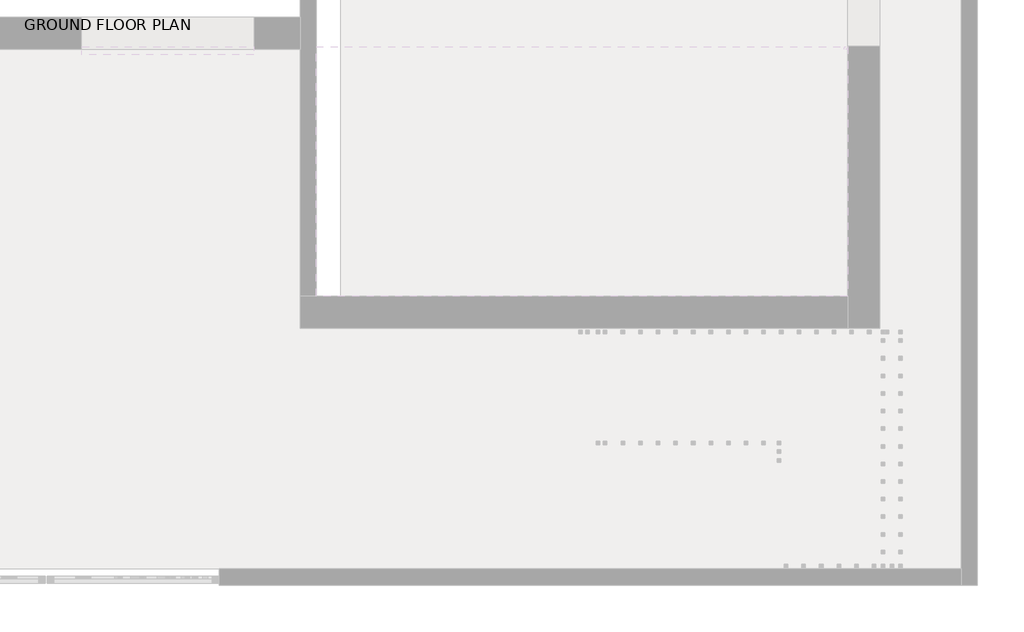
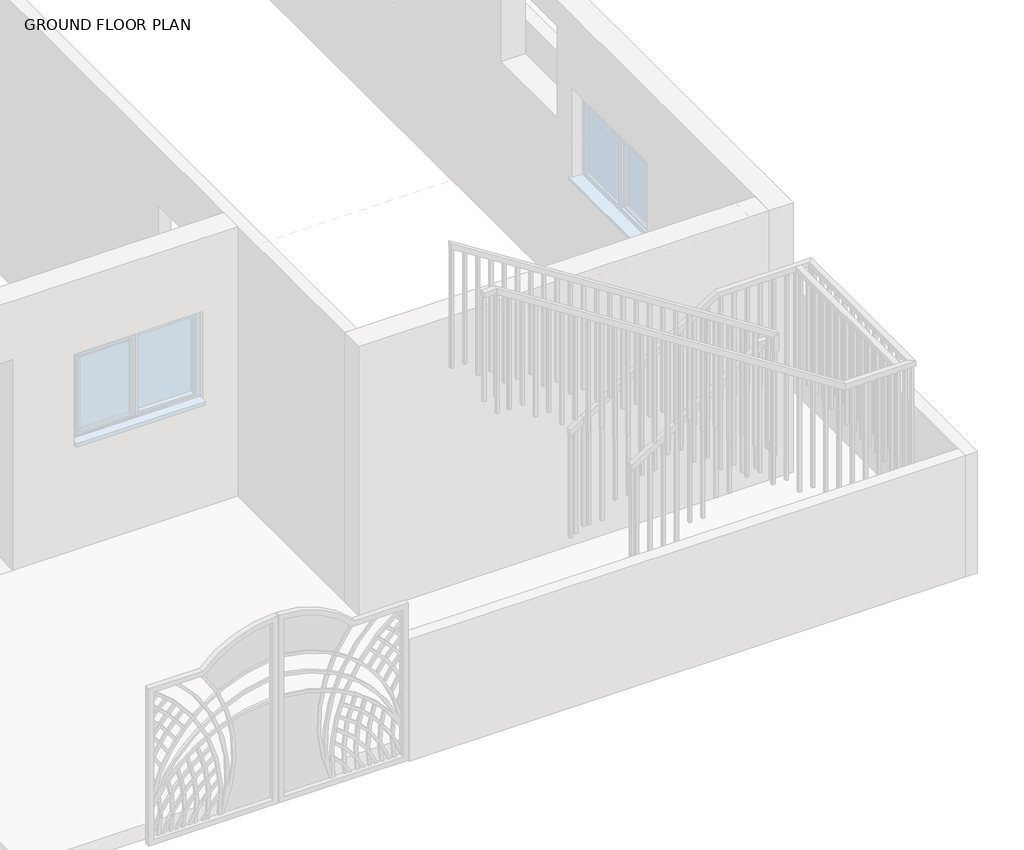
# One storey, part 12 of 23: 2 railings.
"""IFC4 building model written with IfcOpenShell, lengths in millimetres."""

from ifc_helpers import new_model, si_unit, frame, origin, place, context, project, spatial, polyline, outline, extrude, faceted_brep, element, save

model = new_model("IFC4")

# Units and contexts
model_context = context("Model", 3, world=origin())
ifc_project = project(units=[si_unit("LENGTHUNIT", "METRE", prefix="MILLI")], contexts=[model_context])

# Site, building, storey
site = spatial("IfcSite", under=ifc_project)
building = spatial("IfcBuilding", under=site)
storey = spatial("IfcBuildingStorey", under=building, Name="GROUND FLOOR PLAN", Elevation=487.68)

# Railings
placement = place(None, origin())
element("IfcRailing", 1, ObjectType="1100mm", at=placement, inside=storey, context=model_context, shape_type="SolidModel", body=[
    faceted_brep([(-8805.870786, -10220.0521308, 1832.3649576), (-8805.870786, -10220.0521308, 1773.007357), (-8805.870786, -10270.0521308, 1773.007357), (-8805.870786, -10270.0521308, 1832.3649576), (-7409.7306254, -10220.0521308, 2725.6), (-7395.1045513, -10220.0521308, 2675.6), (-7395.1045513, -10270.0521308, 2675.6), (-7409.7306254, -10270.0521308, 2725.6), (-6621.5344696, -10220.0521308, 2725.6), (-6621.5344696, -10220.0521308, 2675.6), (-6671.5344696, -10270.0521308, 2675.6), (-6671.5344696, -10270.0521308, 2725.6), (-6621.5344696, -11933.6860066, 2725.6), (-6621.5344696, -11933.6860066, 2675.6), (-6671.5344696, -11883.6860066, 2675.6), (-6671.5344696, -11883.6860066, 2725.6), (-7155.718398, -11933.6860066, 2725.6), (-7170.3479429, -11933.6860066, 2675.6), (-7170.3479429, -11883.6860066, 2675.6), (-7155.718398, -11883.6860066, 2725.6), (-10457.8773536, -11933.6860066, 4838.88), (-10472.5068984, -11933.6860066, 4788.88), (-10472.5068984, -11883.6860066, 4788.88), (-10457.8773536, -11883.6860066, 4838.88), (-10583.5985666, -11933.6860066, 4838.88), (-10583.5985666, -11883.6860066, 4838.88), (-10583.5985666, -11883.6860066, 4788.88), (-10583.5985666, -11933.6860066, 4788.88)], [[[0, 1, 2, 3]], [[1, 0, 4, 5]], [[2, 1, 5, 6]], [[3, 2, 6, 7]], [[0, 3, 7, 4]], [[5, 4, 8, 9]], [[6, 5, 9, 10]], [[7, 6, 10, 11]], [[4, 7, 11, 8]], [[9, 8, 12, 13]], [[10, 9, 13, 14]], [[11, 10, 14, 15]], [[8, 11, 15, 12]], [[13, 12, 16, 17]], [[14, 13, 17, 18]], [[15, 14, 18, 19]], [[12, 15, 19, 16]], [[17, 16, 20, 21]], [[18, 17, 21, 22]], [[19, 18, 22, 23]], [[16, 19, 23, 20]], [[24, 25, 26, 27]], [[21, 20, 24, 27]], [[22, 21, 27, 26]], [[23, 22, 26, 25]], [[20, 23, 25, 24]]]),
    extrude(outline(polyline([(-10446.5344696, -11921.1860066), (-10471.5344696, -11921.1860066), (-10471.5344696, -11896.1860066), (-10446.5344696, -11896.1860066), (-10446.5344696, -11921.1860066)])), frame((0.0, 0.0, 3738.88), z_axis=(0.0, 0.0, 1.0), x_axis=(1.0, 0.0, 0.0)), (0.0, 0.0, 1.0), 1050.0),
    extrude(outline(polyline([(4692.2622966, -10321.5344696), (4708.2615264, -10346.5344696), (3576.32, -10346.5344696), (3576.32, -10321.5344696), (4692.2622966, -10321.5344696)])), frame((0.0, -11921.1860066, 0.0), z_axis=(0.0, 1.0, 0.0), x_axis=(0.0, 0.0, 1.0)), (0.0, 0.0, 1.0), 25.0),
    extrude(outline(polyline([(4612.2661476, -10196.5344696), (4628.2653774, -10221.5344696), (3576.32, -10221.5344696), (3576.32, -10196.5344696), (4612.2661476, -10196.5344696)])), frame((0.0, -11921.1860066, 0.0), z_axis=(0.0, 1.0, 0.0), x_axis=(0.0, 0.0, 1.0)), (0.0, 0.0, 1.0), 25.0),
    extrude(outline(polyline([(4532.2699985, -10071.5344696), (4548.2692283, -10096.5344696), (3413.76, -10096.5344696), (3413.76, -10071.5344696), (4532.2699985, -10071.5344696)])), frame((0.0, -11921.1860066, 0.0), z_axis=(0.0, 1.0, 0.0), x_axis=(0.0, 0.0, 1.0)), (0.0, 0.0, 1.0), 25.0),
    extrude(outline(polyline([(4452.2738495, -9946.5344696), (4468.2730793, -9971.5344696), (3413.76, -9971.5344696), (3413.76, -9946.5344696), (4452.2738495, -9946.5344696)])), frame((0.0, -11921.1860066, 0.0), z_axis=(0.0, 1.0, 0.0), x_axis=(0.0, 0.0, 1.0)), (0.0, 0.0, 1.0), 25.0),
    extrude(outline(polyline([(4372.2777004, -9821.5344696), (4388.2769302, -9846.5344696), (3251.2, -9846.5344696), (3251.2, -9821.5344696), (4372.2777004, -9821.5344696)])), frame((0.0, -11921.1860066, 0.0), z_axis=(0.0, 1.0, 0.0), x_axis=(0.0, 0.0, 1.0)), (0.0, 0.0, 1.0), 25.0),
    extrude(outline(polyline([(4292.2815514, -9696.5344696), (4308.2807812, -9721.5344696), (3251.2, -9721.5344696), (3251.2, -9696.5344696), (4292.2815514, -9696.5344696)])), frame((0.0, -11921.1860066, 0.0), z_axis=(0.0, 1.0, 0.0), x_axis=(0.0, 0.0, 1.0)), (0.0, 0.0, 1.0), 25.0),
    extrude(outline(polyline([(4212.2854023, -9571.5344696), (4228.2846321, -9596.5344696), (3088.64, -9596.5344696), (3088.64, -9571.5344696), (4212.2854023, -9571.5344696)])), frame((0.0, -11921.1860066, 0.0), z_axis=(0.0, 1.0, 0.0), x_axis=(0.0, 0.0, 1.0)), (0.0, 0.0, 1.0), 25.0),
    extrude(outline(polyline([(4132.2892533, -9446.5344696), (4148.2884831, -9471.5344696), (3088.64, -9471.5344696), (3088.64, -9446.5344696), (4132.2892533, -9446.5344696)])), frame((0.0, -11921.1860066, 0.0), z_axis=(0.0, 1.0, 0.0), x_axis=(0.0, 0.0, 1.0)), (0.0, 0.0, 1.0), 25.0),
    extrude(outline(polyline([(4052.2931042, -9321.5344696), (4068.292334, -9346.5344696), (2926.08, -9346.5344696), (2926.08, -9321.5344696), (4052.2931042, -9321.5344696)])), frame((0.0, -11921.1860066, 0.0), z_axis=(0.0, 1.0, 0.0), x_axis=(0.0, 0.0, 1.0)), (0.0, 0.0, 1.0), 25.0),
    extrude(outline(polyline([(3972.2969552, -9196.5344696), (3988.296185, -9221.5344696), (2926.08, -9221.5344696), (2926.08, -9196.5344696), (3972.2969552, -9196.5344696)])), frame((0.0, -11921.1860066, 0.0), z_axis=(0.0, 1.0, 0.0), x_axis=(0.0, 0.0, 1.0)), (0.0, 0.0, 1.0), 25.0),
    extrude(outline(polyline([(3892.3008061, -9071.5344696), (3908.3000359, -9096.5344696), (2763.52, -9096.5344696), (2763.52, -9071.5344696), (3892.3008061, -9071.5344696)])), frame((0.0, -11921.1860066, 0.0), z_axis=(0.0, 1.0, 0.0), x_axis=(0.0, 0.0, 1.0)), (0.0, 0.0, 1.0), 25.0),
    extrude(outline(polyline([(3812.3046571, -8946.5344696), (3828.3038869, -8971.5344696), (2763.52, -8971.5344696), (2763.52, -8946.5344696), (3812.3046571, -8946.5344696)])), frame((0.0, -11921.1860066, 0.0), z_axis=(0.0, 1.0, 0.0), x_axis=(0.0, 0.0, 1.0)), (0.0, 0.0, 1.0), 25.0),
    extrude(outline(polyline([(3732.308508, -8821.5344696), (3748.3077378, -8846.5344696), (2600.96, -8846.5344696), (2600.96, -8821.5344696), (3732.308508, -8821.5344696)])), frame((0.0, -11921.1860066, 0.0), z_axis=(0.0, 1.0, 0.0), x_axis=(0.0, 0.0, 1.0)), (0.0, 0.0, 1.0), 25.0),
    extrude(outline(polyline([(3652.312359, -8696.5344696), (3668.3115888, -8721.5344696), (2600.96, -8721.5344696), (2600.96, -8696.5344696), (3652.312359, -8696.5344696)])), frame((0.0, -11921.1860066, 0.0), z_axis=(0.0, 1.0, 0.0), x_axis=(0.0, 0.0, 1.0)), (0.0, 0.0, 1.0), 25.0),
    extrude(outline(polyline([(3572.3162099, -8571.5344696), (3588.3154397, -8596.5344696), (2438.4, -8596.5344696), (2438.4, -8571.5344696), (3572.3162099, -8571.5344696)])), frame((0.0, -11921.1860066, 0.0), z_axis=(0.0, 1.0, 0.0), x_axis=(0.0, 0.0, 1.0)), (0.0, 0.0, 1.0), 25.0),
    extrude(outline(polyline([(3492.3200609, -8446.5344696), (3508.3192907, -8471.5344696), (2438.4, -8471.5344696), (2438.4, -8446.5344696), (3492.3200609, -8446.5344696)])), frame((0.0, -11921.1860066, 0.0), z_axis=(0.0, 1.0, 0.0), x_axis=(0.0, 0.0, 1.0)), (0.0, 0.0, 1.0), 25.0),
    extrude(outline(polyline([(3412.3239118, -8321.5344696), (3428.3231416, -8346.5344696), (2275.84, -8346.5344696), (2275.84, -8321.5344696), (3412.3239118, -8321.5344696)])), frame((0.0, -11921.1860066, 0.0), z_axis=(0.0, 1.0, 0.0), x_axis=(0.0, 0.0, 1.0)), (0.0, 0.0, 1.0), 25.0),
    extrude(outline(polyline([(3332.3277628, -8196.5344696), (3348.3269926, -8221.5344696), (2275.84, -8221.5344696), (2275.84, -8196.5344696), (3332.3277628, -8196.5344696)])), frame((0.0, -11921.1860066, 0.0), z_axis=(0.0, 1.0, 0.0), x_axis=(0.0, 0.0, 1.0)), (0.0, 0.0, 1.0), 25.0),
    extrude(outline(polyline([(3252.3316137, -8071.5344696), (3268.3308435, -8096.5344696), (2113.28, -8096.5344696), (2113.28, -8071.5344696), (3252.3316137, -8071.5344696)])), frame((0.0, -11921.1860066, 0.0), z_axis=(0.0, 1.0, 0.0), x_axis=(0.0, 0.0, 1.0)), (0.0, 0.0, 1.0), 25.0),
    extrude(outline(polyline([(3172.3354647, -7946.5344696), (3188.3346945, -7971.5344696), (2113.28, -7971.5344696), (2113.28, -7946.5344696), (3172.3354647, -7946.5344696)])), frame((0.0, -11921.1860066, 0.0), z_axis=(0.0, 1.0, 0.0), x_axis=(0.0, 0.0, 1.0)), (0.0, 0.0, 1.0), 25.0),
    extrude(outline(polyline([(3092.4129874, -7821.5344696), (3108.4077111, -7846.5344696), (1950.72, -7846.5344696), (1950.72, -7821.5344696), (3092.4129874, -7821.5344696)])), frame((0.0, -11921.1860066, 0.0), z_axis=(0.0, 1.0, 0.0), x_axis=(0.0, 0.0, 1.0)), (0.0, 0.0, 1.0), 25.0),
    extrude(outline(polyline([(3012.4393691, -7696.5344696), (3028.4340928, -7721.5344696), (1950.72, -7721.5344696), (1950.72, -7696.5344696), (3012.4393691, -7696.5344696)])), frame((0.0, -11921.1860066, 0.0), z_axis=(0.0, 1.0, 0.0), x_axis=(0.0, 0.0, 1.0)), (0.0, 0.0, 1.0), 25.0),
    extrude(outline(polyline([(2932.4657508, -7571.5344696), (2948.4604745, -7596.5344696), (1788.16, -7596.5344696), (1788.16, -7571.5344696), (2932.4657508, -7571.5344696)])), frame((0.0, -11921.1860066, 0.0), z_axis=(0.0, 1.0, 0.0), x_axis=(0.0, 0.0, 1.0)), (0.0, 0.0, 1.0), 25.0),
    extrude(outline(polyline([(2852.4921325, -7446.5344696), (2868.4868562, -7471.5344696), (1788.16, -7471.5344696), (1788.16, -7446.5344696), (2852.4921325, -7446.5344696)])), frame((0.0, -11921.1860066, 0.0), z_axis=(0.0, 1.0, 0.0), x_axis=(0.0, 0.0, 1.0)), (0.0, 0.0, 1.0), 25.0),
    extrude(outline(polyline([(2772.3547194, -7321.5344696), (2788.3539492, -7346.5344696), (1625.6, -7346.5344696), (1625.6, -7321.5344696), (2772.3547194, -7321.5344696)])), frame((0.0, -11921.1860066, 0.0), z_axis=(0.0, 1.0, 0.0), x_axis=(0.0, 0.0, 1.0)), (0.0, 0.0, 1.0), 25.0),
    extrude(outline(polyline([(2692.3585703, -7196.5344696), (2708.3578001, -7221.5344696), (1625.6, -7221.5344696), (1625.6, -7196.5344696), (2692.3585703, -7196.5344696)])), frame((0.0, -11921.1860066, 0.0), z_axis=(0.0, 1.0, 0.0), x_axis=(0.0, 0.0, 1.0)), (0.0, 0.0, 1.0), 25.0),
    extrude(outline(polyline([(-7071.5344696, -11921.1860066), (-7096.5344696, -11921.1860066), (-7096.5344696, -11896.1860066), (-7071.5344696, -11896.1860066), (-7071.5344696, -11921.1860066)])), frame((0.0, 0.0, 1625.6), z_axis=(0.0, 0.0, 1.0), x_axis=(1.0, 0.0, 0.0)), (0.0, 0.0, 1.0), 1050.0),
    extrude(outline(polyline([(-6946.5344696, -11921.1860066), (-6971.5344696, -11921.1860066), (-6971.5344696, -11896.1860066), (-6946.5344696, -11896.1860066), (-6946.5344696, -11921.1860066)])), frame((0.0, 0.0, 1625.6), z_axis=(0.0, 0.0, 1.0), x_axis=(1.0, 0.0, 0.0)), (0.0, 0.0, 1.0), 1050.0),
    extrude(outline(polyline([(-6821.5344696, -11921.1860066), (-6846.5344696, -11921.1860066), (-6846.5344696, -11896.1860066), (-6821.5344696, -11896.1860066), (-6821.5344696, -11921.1860066)])), frame((0.0, 0.0, 1625.6), z_axis=(0.0, 0.0, 1.0), x_axis=(1.0, 0.0, 0.0)), (0.0, 0.0, 1.0), 1050.0),
    extrude(outline(polyline([(-6696.5344696, -11921.1860066), (-6721.5344696, -11921.1860066), (-6721.5344696, -11896.1860066), (-6696.5344696, -11896.1860066), (-6696.5344696, -11921.1860066)])), frame((0.0, 0.0, 1625.6), z_axis=(0.0, 0.0, 1.0), x_axis=(1.0, 0.0, 0.0)), (0.0, 0.0, 1.0), 1050.0),
    extrude(outline(polyline([(-6634.0344696, -11795.0521308), (-6634.0344696, -11820.0521308), (-6659.0344696, -11820.0521308), (-6659.0344696, -11795.0521308), (-6634.0344696, -11795.0521308)])), frame((0.0, 0.0, 1625.6), z_axis=(0.0, 0.0, 1.0), x_axis=(1.0, 0.0, 0.0)), (0.0, 0.0, 1.0), 1050.0),
    extrude(outline(polyline([(-6634.0344696, -11670.0521308), (-6634.0344696, -11695.0521308), (-6659.0344696, -11695.0521308), (-6659.0344696, -11670.0521308), (-6634.0344696, -11670.0521308)])), frame((0.0, 0.0, 1625.6), z_axis=(0.0, 0.0, 1.0), x_axis=(1.0, 0.0, 0.0)), (0.0, 0.0, 1.0), 1050.0),
    extrude(outline(polyline([(-6634.0344696, -11545.0521308), (-6634.0344696, -11570.0521308), (-6659.0344696, -11570.0521308), (-6659.0344696, -11545.0521308), (-6634.0344696, -11545.0521308)])), frame((0.0, 0.0, 1625.6), z_axis=(0.0, 0.0, 1.0), x_axis=(1.0, 0.0, 0.0)), (0.0, 0.0, 1.0), 1050.0),
    extrude(outline(polyline([(-6634.0344696, -11420.0521308), (-6634.0344696, -11445.0521308), (-6659.0344696, -11445.0521308), (-6659.0344696, -11420.0521308), (-6634.0344696, -11420.0521308)])), frame((0.0, 0.0, 1625.6), z_axis=(0.0, 0.0, 1.0), x_axis=(1.0, 0.0, 0.0)), (0.0, 0.0, 1.0), 1050.0),
    extrude(outline(polyline([(-6634.0344696, -11295.0521308), (-6634.0344696, -11320.0521308), (-6659.0344696, -11320.0521308), (-6659.0344696, -11295.0521308), (-6634.0344696, -11295.0521308)])), frame((0.0, 0.0, 1625.6), z_axis=(0.0, 0.0, 1.0), x_axis=(1.0, 0.0, 0.0)), (0.0, 0.0, 1.0), 1050.0),
    extrude(outline(polyline([(-6634.0344696, -11170.0521308), (-6634.0344696, -11195.0521308), (-6659.0344696, -11195.0521308), (-6659.0344696, -11170.0521308), (-6634.0344696, -11170.0521308)])), frame((0.0, 0.0, 1625.6), z_axis=(0.0, 0.0, 1.0), x_axis=(1.0, 0.0, 0.0)), (0.0, 0.0, 1.0), 1050.0),
    extrude(outline(polyline([(-6634.0344696, -11045.0521308), (-6634.0344696, -11070.0521308), (-6659.0344696, -11070.0521308), (-6659.0344696, -11045.0521308), (-6634.0344696, -11045.0521308)])), frame((0.0, 0.0, 1625.6), z_axis=(0.0, 0.0, 1.0), x_axis=(1.0, 0.0, 0.0)), (0.0, 0.0, 1.0), 1050.0),
    extrude(outline(polyline([(-6634.0344696, -10920.0521308), (-6634.0344696, -10945.0521308), (-6659.0344696, -10945.0521308), (-6659.0344696, -10920.0521308), (-6634.0344696, -10920.0521308)])), frame((0.0, 0.0, 1625.6), z_axis=(0.0, 0.0, 1.0), x_axis=(1.0, 0.0, 0.0)), (0.0, 0.0, 1.0), 1050.0),
    extrude(outline(polyline([(-6634.0344696, -10795.0521308), (-6634.0344696, -10820.0521308), (-6659.0344696, -10820.0521308), (-6659.0344696, -10795.0521308), (-6634.0344696, -10795.0521308)])), frame((0.0, 0.0, 1625.6), z_axis=(0.0, 0.0, 1.0), x_axis=(1.0, 0.0, 0.0)), (0.0, 0.0, 1.0), 1050.0),
    extrude(outline(polyline([(-6634.0344696, -10670.0521308), (-6634.0344696, -10695.0521308), (-6659.0344696, -10695.0521308), (-6659.0344696, -10670.0521308), (-6634.0344696, -10670.0521308)])), frame((0.0, 0.0, 1625.6), z_axis=(0.0, 0.0, 1.0), x_axis=(1.0, 0.0, 0.0)), (0.0, 0.0, 1.0), 1050.0),
    extrude(outline(polyline([(-6634.0344696, -10545.0521308), (-6634.0344696, -10570.0521308), (-6659.0344696, -10570.0521308), (-6659.0344696, -10545.0521308), (-6634.0344696, -10545.0521308)])), frame((0.0, 0.0, 1625.6), z_axis=(0.0, 0.0, 1.0), x_axis=(1.0, 0.0, 0.0)), (0.0, 0.0, 1.0), 1050.0),
    extrude(outline(polyline([(-6634.0344696, -10420.0521308), (-6634.0344696, -10445.0521308), (-6659.0344696, -10445.0521308), (-6659.0344696, -10420.0521308), (-6634.0344696, -10420.0521308)])), frame((0.0, 0.0, 1625.6), z_axis=(0.0, 0.0, 1.0), x_axis=(1.0, 0.0, 0.0)), (0.0, 0.0, 1.0), 1050.0),
    extrude(outline(polyline([(-6634.0344696, -10295.0521308), (-6634.0344696, -10320.0521308), (-6659.0344696, -10320.0521308), (-6659.0344696, -10295.0521308), (-6634.0344696, -10295.0521308)])), frame((0.0, 0.0, 1625.6), z_axis=(0.0, 0.0, 1.0), x_axis=(1.0, 0.0, 0.0)), (0.0, 0.0, 1.0), 1050.0),
    extrude(outline(polyline([(-6755.870786, -10232.5521308), (-6730.870786, -10232.5521308), (-6730.870786, -10257.5521308), (-6755.870786, -10257.5521308), (-6755.870786, -10232.5521308)])), frame((0.0, 0.0, 1625.6), z_axis=(0.0, 0.0, 1.0), x_axis=(1.0, 0.0, 0.0)), (0.0, 0.0, 1.0), 1050.0),
    extrude(outline(polyline([(-6880.870786, -10232.5521308), (-6855.870786, -10232.5521308), (-6855.870786, -10257.5521308), (-6880.870786, -10257.5521308), (-6880.870786, -10232.5521308)])), frame((0.0, 0.0, 1625.6), z_axis=(0.0, 0.0, 1.0), x_axis=(1.0, 0.0, 0.0)), (0.0, 0.0, 1.0), 1050.0),
    extrude(outline(polyline([(-7005.870786, -10232.5521308), (-6980.870786, -10232.5521308), (-6980.870786, -10257.5521308), (-7005.870786, -10257.5521308), (-7005.870786, -10232.5521308)])), frame((0.0, 0.0, 1625.6), z_axis=(0.0, 0.0, 1.0), x_axis=(1.0, 0.0, 0.0)), (0.0, 0.0, 1.0), 1050.0),
    extrude(outline(polyline([(-7130.870786, -10232.5521308), (-7105.870786, -10232.5521308), (-7105.870786, -10257.5521308), (-7130.870786, -10257.5521308), (-7130.870786, -10232.5521308)])), frame((0.0, 0.0, 1625.6), z_axis=(0.0, 0.0, 1.0), x_axis=(1.0, 0.0, 0.0)), (0.0, 0.0, 1.0), 1050.0),
    extrude(outline(polyline([(-7255.870786, -10232.5521308), (-7230.870786, -10232.5521308), (-7230.870786, -10257.5521308), (-7255.870786, -10257.5521308), (-7255.870786, -10232.5521308)])), frame((0.0, 0.0, 1625.6), z_axis=(0.0, 0.0, 1.0), x_axis=(1.0, 0.0, 0.0)), (0.0, 0.0, 1.0), 1050.0),
    extrude(outline(polyline([(-7380.870786, -10232.5521308), (-7355.870786, -10232.5521308), (-7355.870786, -10257.5521308), (-7380.870786, -10257.5521308), (-7380.870786, -10232.5521308)])), frame((0.0, 0.0, 1625.6), z_axis=(0.0, 0.0, 1.0), x_axis=(1.0, 0.0, 0.0)), (0.0, 0.0, 1.0), 1050.0),
    extrude(outline(polyline([(1463.04, -7505.870786), (1463.04, -7480.870786), (2620.7277111, -7480.870786), (2604.7329874, -7505.870786), (1463.04, -7505.870786)])), frame((0.0, -10257.5521308, 0.0), z_axis=(0.0, 1.0, 0.0), x_axis=(0.0, 0.0, 1.0)), (0.0, 0.0, 1.0), 25.0),
    extrude(outline(polyline([(1463.04, -7630.870786), (1463.04, -7605.870786), (2540.7540928, -7605.870786), (2524.7593691, -7630.870786), (1463.04, -7630.870786)])), frame((0.0, -10257.5521308, 0.0), z_axis=(0.0, 1.0, 0.0), x_axis=(0.0, 0.0, 1.0)), (0.0, 0.0, 1.0), 25.0),
    extrude(outline(polyline([(1300.48, -7755.870786), (1300.48, -7730.870786), (2460.7804745, -7730.870786), (2444.7857508, -7755.870786), (1300.48, -7755.870786)])), frame((0.0, -10257.5521308, 0.0), z_axis=(0.0, 1.0, 0.0), x_axis=(0.0, 0.0, 1.0)), (0.0, 0.0, 1.0), 25.0),
    extrude(outline(polyline([(1300.48, -7880.870786), (1300.48, -7855.870786), (2380.8068562, -7855.870786), (2364.8121325, -7880.870786), (1300.48, -7880.870786)])), frame((0.0, -10257.5521308, 0.0), z_axis=(0.0, 1.0, 0.0), x_axis=(0.0, 0.0, 1.0)), (0.0, 0.0, 1.0), 25.0),
    extrude(outline(polyline([(1137.92, -8005.870786), (1137.92, -7980.870786), (2300.8332379, -7980.870786), (2284.8385142, -8005.870786), (1137.92, -8005.870786)])), frame((0.0, -10257.5521308, 0.0), z_axis=(0.0, 1.0, 0.0), x_axis=(0.0, 0.0, 1.0)), (0.0, 0.0, 1.0), 25.0),
    extrude(outline(polyline([(1137.92, -8130.870786), (1137.92, -8105.870786), (2220.8596196, -8105.870786), (2204.8648959, -8130.870786), (1137.92, -8130.870786)])), frame((0.0, -10257.5521308, 0.0), z_axis=(0.0, 1.0, 0.0), x_axis=(0.0, 0.0, 1.0)), (0.0, 0.0, 1.0), 25.0),
    extrude(outline(polyline([(975.36, -8255.870786), (975.36, -8230.870786), (2140.8860012, -8230.870786), (2124.8912776, -8255.870786), (975.36, -8255.870786)])), frame((0.0, -10257.5521308, 0.0), z_axis=(0.0, 1.0, 0.0), x_axis=(0.0, 0.0, 1.0)), (0.0, 0.0, 1.0), 25.0),
    extrude(outline(polyline([(975.36, -8380.870786), (975.36, -8355.870786), (2060.9123829, -8355.870786), (2044.9176593, -8380.870786), (975.36, -8380.870786)])), frame((0.0, -10257.5521308, 0.0), z_axis=(0.0, 1.0, 0.0), x_axis=(0.0, 0.0, 1.0)), (0.0, 0.0, 1.0), 25.0),
    extrude(outline(polyline([(812.8, -8505.870786), (812.8, -8480.870786), (1980.9387646, -8480.870786), (1964.944041, -8505.870786), (812.8, -8505.870786)])), frame((0.0, -10257.5521308, 0.0), z_axis=(0.0, 1.0, 0.0), x_axis=(0.0, 0.0, 1.0)), (0.0, 0.0, 1.0), 25.0),
    extrude(outline(polyline([(812.8, -8630.870786), (812.8, -8605.870786), (1900.9651463, -8605.870786), (1884.9704227, -8630.870786), (812.8, -8630.870786)])), frame((0.0, -10257.5521308, 0.0), z_axis=(0.0, 1.0, 0.0), x_axis=(0.0, 0.0, 1.0)), (0.0, 0.0, 1.0), 25.0),
    extrude(outline(polyline([(772.3517667, -8755.870786), (772.3517667, -8730.870786), (1820.991528, -8730.870786), (1804.9968044, -8755.870786), (772.3517667, -8755.870786)])), frame((0.0, -10257.5521308, 0.0), z_axis=(0.0, 1.0, 0.0), x_axis=(0.0, 0.0, 1.0)), (0.0, 0.0, 1.0), 25.0),
    extrude(outline(polyline([(-6634.0344696, -11896.1860066), (-6634.0344696, -11921.1860066), (-6659.0344696, -11921.1860066), (-6659.0344696, -11896.1860066), (-6634.0344696, -11896.1860066)])), frame((0.0, 0.0, 1625.6), z_axis=(0.0, 0.0, 1.0), x_axis=(1.0, 0.0, 0.0)), (0.0, 0.0, 1.0), 1050.0),
    extrude(outline(polyline([(-6659.0344696, -10232.5521308), (-6634.0344696, -10232.5521308), (-6634.0344696, -10257.5521308), (-6659.0344696, -10257.5521308), (-6659.0344696, -10232.5521308)])), frame((0.0, 0.0, 1625.6), z_axis=(0.0, 0.0, 1.0), x_axis=(1.0, 0.0, 0.0)), (0.0, 0.0, 1.0), 1050.0),
    extrude(outline(polyline([(-10558.5985666, -11921.1860066), (-10583.5985666, -11921.1860066), (-10583.5985666, -11896.1860066), (-10558.5985666, -11896.1860066), (-10558.5985666, -11921.1860066)])), frame((0.0, 0.0, 3738.88), z_axis=(0.0, 0.0, 1.0), x_axis=(1.0, 0.0, 0.0)), (0.0, 0.0, 1.0), 1050.0),
    extrude(outline(polyline([(740.3623194, -8805.870786), (740.3623194, -8780.870786), (1789.0020807, -8780.870786), (1773.007357, -8805.870786), (740.3623194, -8805.870786)])), frame((0.0, -10257.5521308, 0.0), z_axis=(0.0, 1.0, 0.0), x_axis=(0.0, 0.0, 1.0)), (0.0, 0.0, 1.0), 25.0),
])
element("IfcRailing", 2, ObjectType="1100mm", at=placement, inside=storey, context=model_context, shape_type="SolidModel", body=[
    faceted_brep([(-8680.149573, -11007.9255223, 1912.8), (-8680.149573, -11007.9255223, 1853.4423995), (-8680.149573, -11057.9255223, 1853.4423995), (-8680.149573, -11057.9255223, 1912.8), (-7484.3306254, -11007.9255223, 2677.8717446), (-7434.3306254, -11007.9255223, 2650.5035914), (-7434.3306254, -11057.9255223, 2650.5035914), (-7484.3306254, -11057.9255223, 2677.8717446), (-7484.3306254, -11007.9255223, 2725.6), (-7434.3306254, -11007.9255223, 2675.6), (-7434.3306254, -11057.9255223, 2675.6), (-7484.3306254, -11057.9255223, 2725.6), (-7359.3306254, -11007.9255223, 2725.6), (-7359.3306254, -11007.9255223, 2675.6), (-7409.3306254, -11057.9255223, 2675.6), (-7409.3306254, -11057.9255223, 2725.6), (-7359.3306254, -11132.9255223, 2725.6), (-7359.3306254, -11132.9255223, 2675.6), (-7409.3306254, -11132.9255223, 2675.6), (-7409.3306254, -11132.9255223, 2725.6), (-7359.3306254, -11134.9255223, 2725.6), (-7409.3306254, -11134.9255223, 2725.6), (-7409.3306254, -11184.9255223, 2675.6), (-7359.3306254, -11184.9255223, 2675.6)], [[[0, 1, 2, 3]], [[1, 0, 4, 5]], [[2, 1, 5, 6]], [[3, 2, 6, 7]], [[0, 3, 7, 4]], [[5, 4, 8, 9]], [[6, 5, 9, 10]], [[7, 6, 10, 11]], [[4, 7, 11, 8]], [[9, 8, 12, 13]], [[10, 9, 13, 14]], [[11, 10, 14, 15]], [[8, 11, 15, 12]], [[13, 12, 16, 17]], [[14, 13, 17, 18]], [[15, 14, 18, 19]], [[12, 15, 19, 16]], [[20, 21, 22, 23]], [[17, 16, 20, 23]], [[18, 17, 23, 22]], [[19, 18, 22, 21]], [[16, 19, 21, 20]]]),
    faceted_brep([(-7359.3306254, -11134.9255223, 2725.6), (-7359.3306254, -11184.9255223, 2675.6), (-7409.3306254, -11184.9255223, 2675.6), (-7409.3306254, -11134.9255223, 2725.6), (-7359.3306254, -11134.9255223, 2855.9055527), (-7409.3306254, -11134.9255223, 2828.5415543), (-7409.3306254, -11184.9255223, 2828.5415543), (-7359.3306254, -11184.9255223, 2855.9055527)], [[[0, 1, 2, 3]], [[4, 5, 6, 7]], [[1, 0, 4, 7]], [[2, 1, 7, 6]], [[3, 2, 6, 5]], [[0, 3, 5, 4]]]),
    faceted_brep([(-7359.3306254, -11184.9255223, 2855.9055527), (-7409.3306254, -11184.9255223, 2828.5415543), (-7409.3306254, -11134.9255223, 2828.5415543), (-7359.3306254, -11134.9255223, 2855.9055527), (-10457.8773536, -11184.9255223, 4838.88), (-10457.8773536, -11134.9255223, 4838.88), (-10457.8773536, -11134.9255223, 4779.517542), (-10457.8773536, -11184.9255223, 4779.517542)], [[[0, 1, 2, 3]], [[4, 5, 6, 7]], [[1, 0, 4, 7]], [[2, 1, 7, 6]], [[3, 2, 6, 5]], [[0, 3, 5, 4]]]),
    extrude(outline(polyline([(3576.32, -10434.3306254), (4764.4483614, -10434.3306254), (4780.4475912, -10459.3306254), (3576.32, -10459.3306254), (3576.32, -10434.3306254)])), frame((0.0, -11172.4255223, 0.0), z_axis=(0.0, 1.0, 0.0), x_axis=(0.0, 0.0, 1.0)), (0.0, 0.0, 1.0), 25.0),
    extrude(outline(polyline([(3576.32, -10309.3306254), (4684.4522123, -10309.3306254), (4700.4514422, -10334.3306254), (3576.32, -10334.3306254), (3576.32, -10309.3306254)])), frame((0.0, -11172.4255223, 0.0), z_axis=(0.0, 1.0, 0.0), x_axis=(0.0, 0.0, 1.0)), (0.0, 0.0, 1.0), 25.0),
    extrude(outline(polyline([(3413.76, -10184.3306254), (4604.4560633, -10184.3306254), (4620.4552931, -10209.3306254), (3413.76, -10209.3306254), (3413.76, -10184.3306254)])), frame((0.0, -11172.4255223, 0.0), z_axis=(0.0, 1.0, 0.0), x_axis=(0.0, 0.0, 1.0)), (0.0, 0.0, 1.0), 25.0),
    extrude(outline(polyline([(3413.76, -10059.3306254), (4524.4599142, -10059.3306254), (4540.459144, -10084.3306254), (3413.76, -10084.3306254), (3413.76, -10059.3306254)])), frame((0.0, -11172.4255223, 0.0), z_axis=(0.0, 1.0, 0.0), x_axis=(0.0, 0.0, 1.0)), (0.0, 0.0, 1.0), 25.0),
    extrude(outline(polyline([(3251.2, -9934.3306254), (4444.4637652, -9934.3306254), (4460.462995, -9959.3306254), (3251.2, -9959.3306254), (3251.2, -9934.3306254)])), frame((0.0, -11172.4255223, 0.0), z_axis=(0.0, 1.0, 0.0), x_axis=(0.0, 0.0, 1.0)), (0.0, 0.0, 1.0), 25.0),
    extrude(outline(polyline([(3251.2, -9809.3306254), (4364.4676161, -9809.3306254), (4380.4668459, -9834.3306254), (3251.2, -9834.3306254), (3251.2, -9809.3306254)])), frame((0.0, -11172.4255223, 0.0), z_axis=(0.0, 1.0, 0.0), x_axis=(0.0, 0.0, 1.0)), (0.0, 0.0, 1.0), 25.0),
    extrude(outline(polyline([(3251.2, -9684.3306254), (4284.4714671, -9684.3306254), (4300.4706969, -9709.3306254), (3251.2, -9709.3306254), (3251.2, -9684.3306254)])), frame((0.0, -11172.4255223, 0.0), z_axis=(0.0, 1.0, 0.0), x_axis=(0.0, 0.0, 1.0)), (0.0, 0.0, 1.0), 25.0),
    extrude(outline(polyline([(3088.64, -9559.3306254), (4204.475318, -9559.3306254), (4220.4745478, -9584.3306254), (3088.64, -9584.3306254), (3088.64, -9559.3306254)])), frame((0.0, -11172.4255223, 0.0), z_axis=(0.0, 1.0, 0.0), x_axis=(0.0, 0.0, 1.0)), (0.0, 0.0, 1.0), 25.0),
    extrude(outline(polyline([(3088.64, -9434.3306254), (4124.479169, -9434.3306254), (4140.4783988, -9459.3306254), (3088.64, -9459.3306254), (3088.64, -9434.3306254)])), frame((0.0, -11172.4255223, 0.0), z_axis=(0.0, 1.0, 0.0), x_axis=(0.0, 0.0, 1.0)), (0.0, 0.0, 1.0), 25.0),
    extrude(outline(polyline([(2926.08, -9309.3306254), (4044.4830199, -9309.3306254), (4060.4822497, -9334.3306254), (2926.08, -9334.3306254), (2926.08, -9309.3306254)])), frame((0.0, -11172.4255223, 0.0), z_axis=(0.0, 1.0, 0.0), x_axis=(0.0, 0.0, 1.0)), (0.0, 0.0, 1.0), 25.0),
    extrude(outline(polyline([(2926.08, -9184.3306254), (3964.4868709, -9184.3306254), (3980.4861007, -9209.3306254), (2926.08, -9209.3306254), (2926.08, -9184.3306254)])), frame((0.0, -11172.4255223, 0.0), z_axis=(0.0, 1.0, 0.0), x_axis=(0.0, 0.0, 1.0)), (0.0, 0.0, 1.0), 25.0),
    extrude(outline(polyline([(2763.52, -9059.3306254), (3884.4907218, -9059.3306254), (3900.4899516, -9084.3306254), (2763.52, -9084.3306254), (2763.52, -9059.3306254)])), frame((0.0, -11172.4255223, 0.0), z_axis=(0.0, 1.0, 0.0), x_axis=(0.0, 0.0, 1.0)), (0.0, 0.0, 1.0), 25.0),
    extrude(outline(polyline([(2763.52, -8934.3306254), (3804.4945728, -8934.3306254), (3820.4938026, -8959.3306254), (2763.52, -8959.3306254), (2763.52, -8934.3306254)])), frame((0.0, -11172.4255223, 0.0), z_axis=(0.0, 1.0, 0.0), x_axis=(0.0, 0.0, 1.0)), (0.0, 0.0, 1.0), 25.0),
    extrude(outline(polyline([(2600.96, -8809.3306254), (3724.4984237, -8809.3306254), (3740.4976535, -8834.3306254), (2600.96, -8834.3306254), (2600.96, -8809.3306254)])), frame((0.0, -11172.4255223, 0.0), z_axis=(0.0, 1.0, 0.0), x_axis=(0.0, 0.0, 1.0)), (0.0, 0.0, 1.0), 25.0),
    extrude(outline(polyline([(2600.96, -8684.3306254), (3644.5022747, -8684.3306254), (3660.5015045, -8709.3306254), (2600.96, -8709.3306254), (2600.96, -8684.3306254)])), frame((0.0, -11172.4255223, 0.0), z_axis=(0.0, 1.0, 0.0), x_axis=(0.0, 0.0, 1.0)), (0.0, 0.0, 1.0), 25.0),
    extrude(outline(polyline([(2438.4, -8559.3306254), (3564.5061256, -8559.3306254), (3580.5053554, -8584.3306254), (2438.4, -8584.3306254), (2438.4, -8559.3306254)])), frame((0.0, -11172.4255223, 0.0), z_axis=(0.0, 1.0, 0.0), x_axis=(0.0, 0.0, 1.0)), (0.0, 0.0, 1.0), 25.0),
    extrude(outline(polyline([(2438.4, -8434.3306254), (3484.5099766, -8434.3306254), (3500.5092064, -8459.3306254), (2438.4, -8459.3306254), (2438.4, -8434.3306254)])), frame((0.0, -11172.4255223, 0.0), z_axis=(0.0, 1.0, 0.0), x_axis=(0.0, 0.0, 1.0)), (0.0, 0.0, 1.0), 25.0),
    extrude(outline(polyline([(2275.84, -8309.3306254), (3404.5138275, -8309.3306254), (3420.5130573, -8334.3306254), (2275.84, -8334.3306254), (2275.84, -8309.3306254)])), frame((0.0, -11172.4255223, 0.0), z_axis=(0.0, 1.0, 0.0), x_axis=(0.0, 0.0, 1.0)), (0.0, 0.0, 1.0), 25.0),
    extrude(outline(polyline([(2275.84, -8184.3306254), (3324.5176785, -8184.3306254), (3340.5169083, -8209.3306254), (2275.84, -8209.3306254), (2275.84, -8184.3306254)])), frame((0.0, -11172.4255223, 0.0), z_axis=(0.0, 1.0, 0.0), x_axis=(0.0, 0.0, 1.0)), (0.0, 0.0, 1.0), 25.0),
    extrude(outline(polyline([(2113.28, -8059.3306254), (3244.5215294, -8059.3306254), (3260.5207592, -8084.3306254), (2113.28, -8084.3306254), (2113.28, -8059.3306254)])), frame((0.0, -11172.4255223, 0.0), z_axis=(0.0, 1.0, 0.0), x_axis=(0.0, 0.0, 1.0)), (0.0, 0.0, 1.0), 25.0),
    extrude(outline(polyline([(2113.28, -7934.3306254), (3164.5253804, -7934.3306254), (3180.5246102, -7959.3306254), (2113.28, -7959.3306254), (2113.28, -7934.3306254)])), frame((0.0, -11172.4255223, 0.0), z_axis=(0.0, 1.0, 0.0), x_axis=(0.0, 0.0, 1.0)), (0.0, 0.0, 1.0), 25.0),
    extrude(outline(polyline([(1950.72, -7809.3306254), (3084.5292313, -7809.3306254), (3100.5284611, -7834.3306254), (1950.72, -7834.3306254), (1950.72, -7809.3306254)])), frame((0.0, -11172.4255223, 0.0), z_axis=(0.0, 1.0, 0.0), x_axis=(0.0, 0.0, 1.0)), (0.0, 0.0, 1.0), 25.0),
    extrude(outline(polyline([(1950.72, -7684.3306254), (3004.5330823, -7684.3306254), (3020.5323121, -7709.3306254), (1950.72, -7709.3306254), (1950.72, -7684.3306254)])), frame((0.0, -11172.4255223, 0.0), z_axis=(0.0, 1.0, 0.0), x_axis=(0.0, 0.0, 1.0)), (0.0, 0.0, 1.0), 25.0),
    extrude(outline(polyline([(1788.16, -7559.3306254), (2924.5369332, -7559.3306254), (2940.536163, -7584.3306254), (1788.16, -7584.3306254), (1788.16, -7559.3306254)])), frame((0.0, -11172.4255223, 0.0), z_axis=(0.0, 1.0, 0.0), x_axis=(0.0, 0.0, 1.0)), (0.0, 0.0, 1.0), 25.0),
    extrude(outline(polyline([(1788.16, -7434.3306254), (2844.5407841, -7434.3306254), (2860.540014, -7459.3306254), (1788.16, -7459.3306254), (1788.16, -7434.3306254)])), frame((0.0, -11172.4255223, 0.0), z_axis=(0.0, 1.0, 0.0), x_axis=(0.0, 0.0, 1.0)), (0.0, 0.0, 1.0), 25.0),
    extrude(outline(polyline([(-7396.8306254, -11082.9255223), (-7371.8306254, -11082.9255223), (-7371.8306254, -11107.9255223), (-7396.8306254, -11107.9255223), (-7396.8306254, -11082.9255223)])), frame((0.0, 0.0, 1625.6), z_axis=(0.0, 0.0, 1.0), x_axis=(1.0, 0.0, 0.0)), (0.0, 0.0, 1.0), 1050.0),
    extrude(outline(polyline([(2605.1944115, -7505.149573), (1463.04, -7505.149573), (1463.04, -7480.149573), (2621.1891352, -7480.149573), (2605.1944115, -7505.149573)])), frame((0.0, -11045.4255223, 0.0), z_axis=(0.0, 1.0, 0.0), x_axis=(0.0, 0.0, 1.0)), (0.0, 0.0, 1.0), 25.0),
    extrude(outline(polyline([(2525.2207932, -7630.149573), (1463.04, -7630.149573), (1463.04, -7605.149573), (2541.2155169, -7605.149573), (2525.2207932, -7630.149573)])), frame((0.0, -11045.4255223, 0.0), z_axis=(0.0, 1.0, 0.0), x_axis=(0.0, 0.0, 1.0)), (0.0, 0.0, 1.0), 25.0),
    extrude(outline(polyline([(2445.2471749, -7755.149573), (1300.48, -7755.149573), (1300.48, -7730.149573), (2461.2418986, -7730.149573), (2445.2471749, -7755.149573)])), frame((0.0, -11045.4255223, 0.0), z_axis=(0.0, 1.0, 0.0), x_axis=(0.0, 0.0, 1.0)), (0.0, 0.0, 1.0), 25.0),
    extrude(outline(polyline([(2365.2735566, -7880.149573), (1300.48, -7880.149573), (1300.48, -7855.149573), (2381.2682803, -7855.149573), (2365.2735566, -7880.149573)])), frame((0.0, -11045.4255223, 0.0), z_axis=(0.0, 1.0, 0.0), x_axis=(0.0, 0.0, 1.0)), (0.0, 0.0, 1.0), 25.0),
    extrude(outline(polyline([(2285.2999383, -8005.149573), (1137.92, -8005.149573), (1137.92, -7980.149573), (2301.294662, -7980.149573), (2285.2999383, -8005.149573)])), frame((0.0, -11045.4255223, 0.0), z_axis=(0.0, 1.0, 0.0), x_axis=(0.0, 0.0, 1.0)), (0.0, 0.0, 1.0), 25.0),
    extrude(outline(polyline([(2205.32632, -8130.149573), (1137.92, -8130.149573), (1137.92, -8105.149573), (2221.3210437, -8105.149573), (2205.32632, -8130.149573)])), frame((0.0, -11045.4255223, 0.0), z_axis=(0.0, 1.0, 0.0), x_axis=(0.0, 0.0, 1.0)), (0.0, 0.0, 1.0), 25.0),
    extrude(outline(polyline([(2125.3527017, -8255.149573), (975.36, -8255.149573), (975.36, -8230.149573), (2141.3474254, -8230.149573), (2125.3527017, -8255.149573)])), frame((0.0, -11045.4255223, 0.0), z_axis=(0.0, 1.0, 0.0), x_axis=(0.0, 0.0, 1.0)), (0.0, 0.0, 1.0), 25.0),
    extrude(outline(polyline([(2045.3790834, -8380.149573), (975.36, -8380.149573), (975.36, -8355.149573), (2061.3738071, -8355.149573), (2045.3790834, -8380.149573)])), frame((0.0, -11045.4255223, 0.0), z_axis=(0.0, 1.0, 0.0), x_axis=(0.0, 0.0, 1.0)), (0.0, 0.0, 1.0), 25.0),
    extrude(outline(polyline([(1965.4054651, -8505.149573), (812.8, -8505.149573), (812.8, -8480.149573), (1981.4001888, -8480.149573), (1965.4054651, -8505.149573)])), frame((0.0, -11045.4255223, 0.0), z_axis=(0.0, 1.0, 0.0), x_axis=(0.0, 0.0, 1.0)), (0.0, 0.0, 1.0), 25.0),
    extrude(outline(polyline([(1885.4318468, -8630.149573), (812.8, -8630.149573), (812.8, -8605.149573), (1901.4265705, -8605.149573), (1885.4318468, -8630.149573)])), frame((0.0, -11045.4255223, 0.0), z_axis=(0.0, 1.0, 0.0), x_axis=(0.0, 0.0, 1.0)), (0.0, 0.0, 1.0), 25.0),
    extrude(outline(polyline([(-7396.8306254, -11147.4255223), (-7371.8306254, -11147.4255223), (-7371.8306254, -11172.4255223), (-7396.8306254, -11172.4255223), (-7396.8306254, -11147.4255223)])), frame((0.0, 0.0, 1625.6), z_axis=(0.0, 0.0, 1.0), x_axis=(1.0, 0.0, 0.0)), (0.0, 0.0, 1.0), 1050.0),
    extrude(outline(polyline([(-7396.8306254, -11045.4255223), (-7396.8306254, -11020.4255223), (-7371.8306254, -11020.4255223), (-7371.8306254, -11045.4255223), (-7396.8306254, -11045.4255223)])), frame((0.0, 0.0, 1625.6), z_axis=(0.0, 0.0, 1.0), x_axis=(1.0, 0.0, 0.0)), (0.0, 0.0, 1.0), 1050.0),
    extrude(outline(polyline([(3576.32, -10432.8773536), (4763.5183122, -10432.8773536), (4779.517542, -10457.8773536), (3576.32, -10457.8773536), (3576.32, -10432.8773536)])), frame((0.0, -11172.4255223, 0.0), z_axis=(0.0, 1.0, 0.0), x_axis=(0.0, 0.0, 1.0)), (0.0, 0.0, 1.0), 25.0),
    extrude(outline(polyline([(1853.4423995, -8680.149573), (812.8, -8680.149573), (812.8, -8655.149573), (1869.4371231, -8655.149573), (1853.4423995, -8680.149573)])), frame((0.0, -11045.4255223, 0.0), z_axis=(0.0, 1.0, 0.0), x_axis=(0.0, 0.0, 1.0)), (0.0, 0.0, 1.0), 25.0),
])

save(model, "model.ifc")

# Revit data of these elements
# Type "1100mm"
#   built-in parameter 1008612 = 0.019685 (stored number, unit not read)
#   built-in parameter 1008611 = 0.019685 (stored number, unit not read)
#   built-in parameter 1008609 = 0.902231 (stored number, unit not read)
#   built-in parameter 1008604 = 0.19685 (stored number, unit not read)
#   built-in parameter 1008603 = 0.164042 (stored number, unit not read)
#   Railing Height = 3.608924 ft
#   built-in parameter 1008630 = 2
#   built-in parameter 1008610 = 2
#   built-in parameter 1008608 = 1
#   built-in parameter 1008618 = Baluster_Square : 25mm
# Elements 1, 2 (IfcRailing, "1100mm")
#   Phase Created = New Construction
